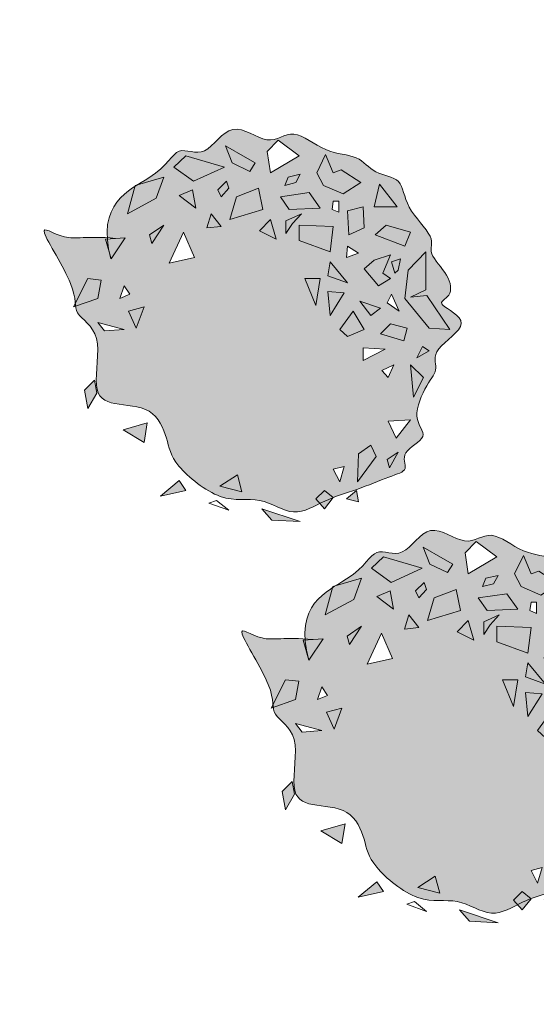
# Model space of a CAD drawing. Units: metres. Extents: x 4298.5 to 4325.2, y 2075 to 2095.8.
# Tile 23 of 35: x 4318.327 to 4319.132, y 2078.198 to 2079.73. Entities that reach past the tile are written whole.
import ezdxf

# ---------------------------------------------------------------- set-up
doc = ezdxf.new("R2010")
doc.units = ezdxf.units.M
doc.layers.add('A-ANNO-DIMS', color=2, linetype='Continuous', lineweight=18)
doc.layers.add('L-PLNT', color=94, linetype='Continuous', lineweight=13)
doc.layers.add('L-PLNT-PATT', color=116, linetype='Continuous', lineweight=13, true_color=0x13823e)
doc.styles.get("Standard").update_dxf_attribs({"font": 'arial.ttf'})
doc.dimstyles.get("Standard").update_dxf_attribs({"dimtxt": 0.18, "dimasz": 0.18, "dimexe": 0.18, "dimexo": 0.0625, "dimgap": 0.09, "dimtad": 0, "dimtih": 1, "dimtoh": 1, "dimdec": 4, "dimzin": 0, "dimdsep": 46, "dimtxsty": 'Standard', "dimcen": 0.09, "dimadec": 0, "dimazin": 0, "dimtfac": 1, "dimtdec": 4, "dimtofl": 0, "dimtmove": 0, "dimatfit": 3, "dimfxl": 1, "dimtolj": 1, "dimtzin": 0, "dimarcsym": 0})

# ---------------------------------------------------------------- blocks, each defined once
blk = doc.blocks.new('*U9')
for points in [[(-2.003, 11.656), (-1.598, 10.618), (-0.518, 10.099), (-0.181, 10.618), (-0.788, 10.964)], [(1.237, 12.003), (0.562, 11.31), (0.764, 10.013), (2.519, 11.051)], [(-4.432, 11.051), (-5.175, 10.359), (-3.96, 9.493), (-2.07, 10.359)], [(4.139, 11.137), (3.599, 10.013), (4.004, 9.234), (5.218, 8.715), (6.298, 9.407), (5.083, 10.186), (4.611, 10.013)], [(-5.782, 9.753), (-7.537, 9.234), (-8.009, 7.504), (-6.255, 8.455)], [(2.586, 9.926), (1.844, 9.753), (1.642, 9.234), (2.316, 9.407)], [(-1.935, 9.493), (-2.475, 8.974), (-2.273, 8.542), (-1.8, 9.061)], [(0.022, 9.061), (-1.328, 8.542), (-1.733, 7.157), (0.292, 7.763)], [(7.446, 9.32), (7.108, 7.936), (8.525, 7.936)], [(-4.837, 8.628), (-3.825, 7.85), (-4.027, 8.974)], [(1.372, 8.542), (3.126, 8.801), (3.801, 7.85), (1.912, 7.763)], [(4.611, 8.282), (4.544, 7.763), (4.949, 7.59), (4.949, 8.282)], [(6.433, 7.936), (5.488, 7.676), (5.556, 6.206), (6.501, 6.638)], [(-2.88, 7.504), (-3.15, 6.638), (-2.273, 6.725)], [(1.709, 6.292), (1.709, 7.071), (2.654, 7.504), (2.114, 6.898)], [(-5.782, 6.811), (-6.659, 6.206), (-6.524, 5.687)], [(0.764, 7.157), (0.089, 6.465), (1.102, 5.946)], [(2.519, 6.811), (2.519, 5.86), (4.409, 5.167), (4.611, 6.725)], [(7.851, 6.811), (7.176, 6.206), (8.998, 5.514), (9.335, 6.379)], [(-4.567, 6.379), (-5.445, 4.475), (-3.892, 4.821)], [(-8.144, 6.033), (-9.359, 5.946), (-9.022, 4.735)], [(5.488, 5.514), (5.421, 4.821), (6.163, 5.081)], [(8.12, 4.994), (7.108, 4.648), (6.501, 4.129), (7.378, 3.091), (8.12, 3.524), (7.648, 3.87)], [(10.28, 5.167), (9.2, 4.043), (8.998, 2.312), (10.482, 0.495), (11.765, 0.409), (10.348, 2.485), (9.335, 2.399), (10.28, 2.831)], [(4.409, 4.562), (4.274, 3.697), (5.488, 3.264)], [(8.728, 4.735), (8.188, 4.562), (8.39, 3.87), (8.593, 4.043)], [(-11.316, 1.793), (-9.831, 2.312), (-9.629, 3.437), (-10.439, 3.524)], [(-8.212, 3.091), (-8.482, 2.312), (-7.874, 2.572)], [(3.531, 1.88), (2.856, 3.524), (3.801, 3.524)], [(4.274, 2.745), (5.286, 2.658), (4.409, 1.274)], [(8.188, 2.572), (7.918, 2.053), (8.66, 1.534)], [(7.513, 1.707), (6.906, 1.274), (6.231, 2.139)], [(-6.997, 1.793), (-7.942, 1.534), (-7.469, 0.495)], [(5.826, 1.534), (5.016, 0.409), (5.488, -0.024), (6.501, 0.409)], [(-8.212, 0.409), (-9.426, 0.322), (-9.831, 0.841)], [(8.12, 0.755), (7.513, 0.149), (8.93, -0.283), (9.133, 0.495)], [(7.783, -0.803), (6.433, -1.495), (6.433, -0.716)], [(10.078, -0.629), (9.74, -1.322), (10.482, -0.889)], [(8.323, -1.754), (7.985, -2.533), (7.581, -2.1)], [(9.335, -1.754), (9.538, -3.744), (10.145, -2.533)], [(-10.034, -2.706), (-10.641, -3.312), (-10.439, -4.436), (-9.899, -3.485)], [(-8.279, -5.734), (-6.794, -5.302), (-6.997, -6.513)], [(9.335, -5.129), (8.458, -6.253), (7.985, -5.215)], [(6.096, -8.935), (6.163, -7.205), (6.906, -6.686), (7.243, -7.378)], [(8.053, -8.07), (8.593, -7.118), (7.918, -7.551)], [(5.286, -7.984), (4.611, -8.157), (5.016, -8.935)], [(-4.837, -8.849), (-4.432, -9.454), (-5.985, -9.801)], [(-2.34, -9.195), (-1.26, -8.503), (-0.99, -9.541)], [(4.071, -9.454), (3.531, -9.974), (4.071, -10.579), (4.611, -9.887)], [(6.028, -9.454), (5.421, -9.974), (6.163, -10.147)], [(-2.543, -10.06), (-3.015, -10.233), (-1.8, -10.666)], [(0.224, -10.579), (0.832, -11.272), (2.586, -11.358)]]:
    blk.add_lwpolyline(points, close=True)
blk = doc.blocks.new('*D47')
at = {"layer": 'A-ANNO-DIMS', "color": 0, "lineweight": -2, "transparency": 16777216}
for p, q in [((4300.4306, 2084.4956), (4300.4306, 2074.9896)), ((4322.8106, 2084.4956), (4322.8106, 2074.9896)), ((4300.6106, 2075.1696), (4311.2252, 2075.1696)), ((4322.6306, 2075.1696), (4312.016, 2075.1696))]:
    blk.add_line(p, q, dxfattribs=at)
at = {"layer": 'A-ANNO-DIMS', "color": 0, "transparency": 16777216}
for points in [[(4300.6106, 2075.1996), (4300.6106, 2075.1396), (4300.4306, 2075.1696)], [(4322.6306, 2075.1996), (4322.6306, 2075.1396), (4322.8106, 2075.1696)]]:
    blk.add_solid(points, dxfattribs=at)
at = {"layer": 'Defpoints', "color": 0, "transparency": 16777216}
for p in [(4300.4306, 2084.5581), (4322.8106, 2084.5581), (4322.8106, 2075.1696)]:
    blk.add_point(p, dxfattribs=at)
at = {"layer": 'A-ANNO-DIMS', "color": 0, "transparency": 16777216, "insert": (4311.6206, 2075.1696), "char_height": 0.18, "attachment_point": 5}
blk.add_mtext('\\A1;22.38', dxfattribs=at)
blk = doc.blocks.new('*D48')
at = {"layer": 'A-ANNO-DIMS', "color": 0, "lineweight": -2, "transparency": 16777216}
for p, q in [((4310.1831, 2094.4781), (4324.7671, 2094.4781)), ((4324.5871, 2094.2981), (4324.5871, 2085.585)), ((4324.5871, 2076.5081), (4324.5871, 2085.2212)), ((4316.8731, 2076.3281), (4324.7671, 2076.3281))]:
    blk.add_line(p, q, dxfattribs=at)
at = {"layer": 'A-ANNO-DIMS', "color": 0, "transparency": 16777216}
for points in [[(4324.5571, 2094.2981), (4324.6171, 2094.2981), (4324.5871, 2094.4781)], [(4324.5571, 2076.5081), (4324.6171, 2076.5081), (4324.5871, 2076.3281)]]:
    blk.add_solid(points, dxfattribs=at)
at = {"layer": 'Defpoints', "color": 0, "transparency": 16777216}
for p in [(4310.1206, 2094.4781), (4316.8106, 2076.3281), (4324.5871, 2076.3281)]:
    blk.add_point(p, dxfattribs=at)
at = {"layer": 'A-ANNO-DIMS', "color": 0, "transparency": 16777216, "insert": (4324.5871, 2085.4031), "char_height": 0.18, "attachment_point": 5}
blk.add_mtext('\\A1;18.15', dxfattribs=at)
blk = doc.blocks.new('*D79')
at = {"layer": 'A-ANNO-DIMS', "color": 0, "lineweight": -2, "transparency": 16777216}
for p, q in [((4313.4743, 2079.7393), (4313.4743, 2079.9193)), ((4313.3843, 2079.8293), (4313.5643, 2079.8293)), ((4320.4622, 2076.981), (4318.0084, 2077.9812)), ((4320.6422, 2076.981), (4320.4622, 2076.981))]:
    blk.add_line(p, q, dxfattribs=at)
at = {"layer": 'A-ANNO-DIMS', "color": 0, "transparency": 16777216}
blk.add_solid([(4318.0197, 2078.009), (4317.9971, 2077.9534), (4317.8417, 2078.0491)], dxfattribs=at)
at = {"layer": 'Defpoints', "color": 0, "transparency": 16777216}
for p in [(4313.4743, 2079.8293), (4317.8417, 2078.0491)]:
    blk.add_point(p, dxfattribs=at)
at = {"layer": 'A-ANNO-DIMS', "color": 0, "transparency": 16777216, "insert": (4321.3169, 2076.981), "char_height": 0.18, "attachment_point": 5}
blk.add_mtext('\\A1;2X R4.716', dxfattribs=at)

msp = doc.modelspace()

# ---------------------------------------------------------------- hatches: boundary and pattern name
at = {"layer": 'L-PLNT-PATT'}
h = msp.add_hatch(color=256, dxfattribs=at)
h.dxf.hatch_style = 1
edge = h.paths.add_edge_path()
edge.add_spline(control_points=[(4318.7946, 2078.9772), (4318.7972, 2078.9785), (4318.8158, 2078.9878), (4318.8516, 2078.9976), (4318.9061, 2079.0208), (4318.9355, 2079.0284), (4318.9167, 2079.0569), (4318.9693, 2079.0811), (4318.9356, 2079.1074), (4318.9626, 2079.1671), (4318.9813, 2079.1866), (4318.9647, 2079.2151), (4319.0389, 2079.26), (4318.969, 2079.2895), (4319.0017, 2079.2972), (4318.9977, 2079.3323), (4318.9596, 2079.3689), (4318.9782, 2079.3883), (4318.9251, 2079.4393), (4318.9251, 2079.4853), (4318.8773, 2079.4887), (4318.8568, 2079.5206), (4318.8036, 2079.5206), (4318.7513, 2079.5659), (4318.7165, 2079.5288), (4318.6558, 2079.5797), (4318.6159, 2079.5096), (4318.5713, 2079.5396), (4318.557, 2079.5002), (4318.5167, 2079.4772), (4318.5103, 2079.4732)], knot_values=[0.818571, 0.818571, 0.818571, 0.818571, 0.97924, 1.97924, 2.97924, 3.97924, 4.97924, 5.97924, 6.97924, 7.97924, 8.97924, 9.97924, 10.97924, 11.97924, 12.97924, 13.97924, 14.97924, 15.97924, 16.97924, 17.97924, 18.97924, 19.97924, 20.97924, 21.97924, 22.97924, 23.97924, 24.97924, 25.97924, 26.97924, 27.16067, 27.16067, 27.16067, 27.16067], degree=3, periodic=0)
edge.add_line((4318.5103, 2079.4732), (4318.5516, 2079.4854))
edge.add_line((4318.5516, 2079.4854), (4318.5396, 2079.4524))
edge.add_line((4318.5396, 2079.4524), (4318.495, 2079.4283))
edge.add_line((4318.495, 2079.4283), (4318.5067, 2079.4709))
edge.add_spline(control_points=[(4318.5067, 2079.4709), (4318.484, 2079.4562), (4318.4607, 2079.4353), (4318.4635, 2079.3909)], knot_values=[0.141368, 0.141368, 0.141368, 0.141368, 0.783694, 0.783694, 0.783694, 0.783694], degree=3, periodic=0)
edge.add_spline(control_points=[(4318.4635, 2079.3909), (4318.4674, 2079.3906), (4318.4717, 2079.3903), (4318.4762, 2079.3898)], knot_values=[40.901028, 40.901028, 40.901028, 40.901028, 41, 41, 41, 41], degree=3, periodic=0)
edge.add_line((4318.4762, 2079.3898), (4318.4916, 2079.3909))
edge.add_line((4318.4916, 2079.3909), (4318.4693, 2079.358))
edge.add_line((4318.4693, 2079.358), (4318.4608, 2079.3887))
edge.add_line((4318.4608, 2079.3887), (4318.4636, 2079.3889))
edge.add_spline(control_points=[(4318.4636, 2079.3889), (4318.4635, 2079.3896), (4318.4635, 2079.3902), (4318.4635, 2079.3909)], knot_values=[0.13204, 0.13204, 0.13204, 0.13204, 0.141368, 0.141368, 0.141368, 0.141368], degree=3, periodic=0)
edge.add_spline(control_points=[(4318.4635, 2079.3909), (4318.4272, 2079.3932), (4318.3956, 2079.3834), (4318.3436, 2079.4253), (4318.4107, 2079.3228), (4318.413, 2079.2959), (4318.4137, 2079.2885)], knot_values=[37.439141, 37.439141, 37.439141, 37.439141, 38.340169, 39.340169, 40.340169, 40.901028, 40.901028, 40.901028, 40.901028], degree=3, periodic=0)
edge.add_line((4318.4137, 2079.2885), (4318.4333, 2079.3272))
edge.add_line((4318.4333, 2079.3272), (4318.4539, 2079.325))
edge.add_line((4318.4539, 2079.325), (4318.4488, 2079.2964))
edge.add_line((4318.4488, 2079.2964), (4318.4141, 2079.2843))
edge.add_spline(control_points=[(4318.4141, 2079.2843), (4318.4146, 2079.2804), (4318.4177, 2079.2668), (4318.4591, 2079.2459), (4318.4376, 2079.1486), (4318.4698, 2079.1297), (4318.5361, 2079.1297), (4318.5588, 2079.076), (4318.5623, 2079.0405), (4318.6433, 2078.9745), (4318.7016, 2078.9912), (4318.752, 2078.9544), (4318.7811, 2078.9703), (4318.7946, 2078.9772)], knot_values=[27.16067, 27.16067, 27.16067, 27.16067, 27.490087, 28.490087, 29.490087, 30.490087, 31.490087, 32.490087, 33.490087, 34.490087, 35.490087, 36.490087, 37.329418, 37.329418, 37.329418, 37.329418], degree=3, periodic=0)
edge.add_line((4318.7946, 2078.9772), (4318.7882, 2078.9843))
edge.add_line((4318.7882, 2078.9843), (4318.8019, 2078.9976))
edge.add_line((4318.8019, 2078.9976), (4318.8156, 2078.9865))
h.paths.add_polyline_path([(4318.771, 2079.3272), (4318.795, 2079.3272), (4318.7882, 2079.2854)], flags=16)
h.paths.add_polyline_path([(4318.807, 2079.3074), (4318.8327, 2079.3052), (4318.8105, 2079.27)], flags=16)
h.paths.add_polyline_path([(4318.5996, 2079.3601), (4318.5602, 2079.3514), (4318.5825, 2079.3997)], flags=16)
h.paths.add_polyline_path([(4318.7265, 2079.3887), (4318.7007, 2079.4019), (4318.7179, 2079.4195)], flags=16)
h.paths.add_polyline_path([(4318.807, 2079.3316), (4318.8105, 2079.3536), (4318.8379, 2079.3206)], flags=16)
h.paths.add_polyline_path([(4318.8259, 2079.2481), (4318.8465, 2079.2766), (4318.8636, 2079.2481), (4318.8379, 2079.2371)], flags=16)
h.paths.add_polyline_path([(4318.7625, 2079.3865), (4318.7625, 2079.4107), (4318.8156, 2079.4085), (4318.8105, 2079.3689)], flags=16)
h.paths.add_polyline_path([(4318.7419, 2079.3975), (4318.7419, 2079.4173), (4318.7659, 2079.4283), (4318.7522, 2079.4129)], flags=16)
h.paths.add_polyline_path([(4318.6407, 2079.4085), (4318.6185, 2079.4063), (4318.6253, 2079.4283)], flags=16)
h.paths.add_polyline_path([(4318.6545, 2079.4195), (4318.6647, 2079.4547), (4318.699, 2079.4678), (4318.7059, 2079.4349)], flags=16)
h.paths.add_polyline_path([(4318.5207, 2079.2832), (4318.5088, 2079.2503), (4318.4967, 2079.2766)], flags=16)
h.paths.add_polyline_path([(4318.8567, 2079.292), (4318.8893, 2079.281), (4318.8739, 2079.27)], flags=16)
h.paths.add_polyline_path([(4318.8362, 2079.3601), (4318.8379, 2079.3777), (4318.855, 2079.3667)], flags=16)
h.paths.add_polyline_path([(4318.747, 2079.4349), (4318.7333, 2079.4547), (4318.7779, 2079.4612), (4318.795, 2079.4371)], flags=16)
h.paths.add_polyline_path([(4318.8619, 2079.2195), (4318.8962, 2079.2173), (4318.8619, 2079.1997)], flags=16)
h.paths.add_polyline_path([(4318.4985, 2079.303), (4318.483, 2079.2964), (4318.4899, 2079.3162)], flags=16)
h.paths.add_polyline_path([(4318.6013, 2079.4371), (4318.5756, 2079.4568), (4318.5962, 2079.4656)], flags=16)
h.paths.add_polyline_path([(4318.5328, 2079.3821), (4318.5293, 2079.3953), (4318.5516, 2079.4107)], flags=16)
h.paths.add_polyline_path([(4318.6407, 2079.4547), (4318.6356, 2079.4656), (4318.6493, 2079.4788), (4318.6528, 2079.4678)], flags=16)
h.paths.add_polyline_path([(4318.8636, 2079.3426), (4318.879, 2079.3557), (4318.9047, 2079.3645), (4318.8927, 2079.336), (4318.9047, 2079.3272), (4318.8859, 2079.3162)], flags=16)
h.paths.add_polyline_path([(4318.4899, 2079.2481), (4318.4591, 2079.2459), (4318.4488, 2079.259)], flags=16)
h.paths.add_polyline_path([(4318.8396, 2079.3953), (4318.8379, 2079.4327), (4318.8619, 2079.4393), (4318.8636, 2079.4063)], flags=16)
h.paths.add_polyline_path([(4318.8893, 2079.2415), (4318.9047, 2079.2569), (4318.9305, 2079.2503), (4318.9253, 2079.2305)], flags=16)
h.paths.add_polyline_path([(4318.8139, 2079.4349), (4318.8156, 2079.448), (4318.8242, 2079.448), (4318.8242, 2079.4305)], flags=16)
h.paths.add_polyline_path([(4318.7402, 2079.4722), (4318.7453, 2079.4854), (4318.7642, 2079.4898), (4318.7573, 2079.4766)], flags=16)
h.paths.add_polyline_path([(4318.8996, 2079.2898), (4318.9064, 2079.303), (4318.9184, 2079.2766)], flags=16)
h.paths.add_polyline_path([(4318.891, 2079.1843), (4318.9099, 2079.1931), (4318.9013, 2079.1733)], flags=16)
h.paths.add_polyline_path([(4318.6853, 2079.4942), (4318.6579, 2079.5074), (4318.6476, 2079.5337), (4318.6785, 2079.5162), (4318.6939, 2079.5074)], flags=16)
h.paths.add_polyline_path([(4318.7179, 2079.492), (4318.7127, 2079.525), (4318.7299, 2079.5426), (4318.7625, 2079.5184)], flags=16)
h.paths.add_polyline_path([(4318.5979, 2079.4788), (4318.567, 2079.5008), (4318.5859, 2079.5184), (4318.6459, 2079.5008)], flags=16)
h.paths.add_polyline_path([(4318.8807, 2079.3953), (4318.8979, 2079.4107), (4318.9356, 2079.3997), (4318.927, 2079.3777)], flags=16)
h.paths.add_polyline_path([(4318.8002, 2079.4722), (4318.7899, 2079.492), (4318.8036, 2079.5206), (4318.8156, 2079.492), (4318.8276, 2079.4964), (4318.8584, 2079.4766), (4318.831, 2079.459)], flags=16)
h.paths.add_polyline_path([(4318.9116, 2079.336), (4318.9064, 2079.3536), (4318.9202, 2079.358), (4318.9167, 2079.3404)], flags=16)
h.paths.add_polyline_path([(4318.927, 2079.2964), (4318.9322, 2079.3404), (4318.9596, 2079.3689), (4318.9596, 2079.3096), (4318.9356, 2079.2986), (4318.9613, 2079.3008), (4318.9973, 2079.2481), (4318.9647, 2079.2503)], flags=16)
h.paths.add_polyline_path([(4318.6665, 2079.0217), (4318.6733, 2078.9953), (4318.639, 2079.0041)], flags=16)
h.paths.add_polyline_path([(4318.879, 2079.4393), (4318.8876, 2079.4744), (4318.915, 2079.4393)], flags=16)
h.paths.add_polyline_path([(4318.9356, 2079.1931), (4318.9562, 2079.1733), (4318.9407, 2079.1426)], flags=16)
h.paths.add_polyline_path([(4318.9459, 2079.2041), (4318.9545, 2079.2217), (4318.9647, 2079.2151)], flags=16)
h.paths.add_polyline_path([(4318.8156, 2079.0305), (4318.8327, 2079.0349), (4318.8259, 2079.0107)], flags=16)
h.paths.add_polyline_path([(4318.9013, 2079.1052), (4318.9356, 2079.1074), (4318.9133, 2079.0789)], flags=16)
h.paths.add_polyline_path([(4318.855, 2079.0547), (4318.8739, 2079.0679), (4318.8824, 2079.0503), (4318.8533, 2079.0107)], flags=16)
h.paths.add_polyline_path([(4318.8996, 2079.0459), (4318.9167, 2079.0569), (4318.903, 2079.0327)], flags=16)
h = msp.add_hatch(color=256, dxfattribs=at)
h.dxf.hatch_style = 1
h.paths.add_polyline_path([(4318.8105, 2079.3689), (4318.8156, 2079.4085), (4318.7625, 2079.4107), (4318.7625, 2079.3865)])
h.paths.add_polyline_path([(4318.8567, 2079.292), (4318.8739, 2079.27), (4318.8893, 2079.281)])
h.paths.add_polyline_path([(4318.8379, 2079.4327), (4318.8396, 2079.3953), (4318.8636, 2079.4063), (4318.8619, 2079.4393)])
h.paths.add_polyline_path([(4318.8584, 2079.4766), (4318.8276, 2079.4964), (4318.8156, 2079.492), (4318.8036, 2079.5206), (4318.7899, 2079.492), (4318.8002, 2079.4722), (4318.831, 2079.459)])
h.paths.add_polyline_path([(4318.7042, 2078.969), (4318.7196, 2078.9514), (4318.7642, 2078.9492)])
h.paths.add_polyline_path([(4318.6853, 2079.4942), (4318.6939, 2079.5074), (4318.6785, 2079.5162), (4318.6476, 2079.5337), (4318.6579, 2079.5074)])
h.paths.add_polyline_path([(4318.5859, 2079.5184), (4318.567, 2079.5008), (4318.5979, 2079.4788), (4318.6459, 2079.5008)])
h.paths.add_polyline_path([(4318.6647, 2079.4547), (4318.6545, 2079.4195), (4318.7059, 2079.4349), (4318.699, 2079.4678)])
h.paths.add_polyline_path([(4318.6528, 2079.4678), (4318.6493, 2079.4788), (4318.6356, 2079.4656), (4318.6407, 2079.4547)])
h.paths.add_polyline_path([(4318.6253, 2079.4283), (4318.6185, 2079.4063), (4318.6407, 2079.4085)])
h.paths.add_polyline_path([(4318.6013, 2079.4371), (4318.5962, 2079.4656), (4318.5756, 2079.4568)])
h.paths.add_polyline_path([(4318.507, 2079.4722), (4318.495, 2079.4283), (4318.5396, 2079.4524), (4318.5516, 2079.4854)])
h.paths.add_polyline_path([(4318.5516, 2079.4107), (4318.5293, 2079.3953), (4318.5328, 2079.3821)])
h.paths.add_polyline_path([(4318.4608, 2079.3887), (4318.4693, 2079.358), (4318.4916, 2079.3909)])
h.paths.add_polyline_path([(4318.411, 2079.2832), (4318.4488, 2079.2964), (4318.4539, 2079.325), (4318.4333, 2079.3272)])
h.paths.add_polyline_path([(4318.5207, 2079.2832), (4318.4967, 2079.2766), (4318.5088, 2079.2503)])
h.paths.add_polyline_path([(4318.447, 2079.1492), (4318.4436, 2079.169), (4318.4282, 2079.1536), (4318.4333, 2079.125)])
h.paths.add_polyline_path([(4318.5259, 2079.103), (4318.4882, 2079.092), (4318.5207, 2079.0723)])
h.paths.add_polyline_path([(4318.5465, 2078.9887), (4318.5859, 2078.9976), (4318.5756, 2079.0129)])
h.paths.add_polyline_path([(4318.6665, 2079.0217), (4318.639, 2079.0041), (4318.6733, 2078.9953)])
h.paths.add_polyline_path([(4318.8019, 2078.9976), (4318.7882, 2078.9843), (4318.8019, 2078.969), (4318.8156, 2078.9866)])
h.paths.add_polyline_path([(4318.8824, 2079.0503), (4318.8739, 2079.0679), (4318.855, 2079.0547), (4318.8533, 2079.0107)])
h.paths.add_polyline_path([(4318.8516, 2078.9976), (4318.8362, 2078.9843), (4318.855, 2078.98)])
h.paths.add_polyline_path([(4318.8996, 2079.0459), (4318.903, 2079.0327), (4318.9167, 2079.0569)])
h.paths.add_polyline_path([(4318.9407, 2079.1426), (4318.9562, 2079.1733), (4318.9356, 2079.1931)])
h.paths.add_polyline_path([(4318.8259, 2079.2481), (4318.8379, 2079.2371), (4318.8636, 2079.2481), (4318.8465, 2079.2766)])
h.paths.add_polyline_path([(4318.9647, 2079.2503), (4318.9973, 2079.2481), (4318.9613, 2079.3008), (4318.9356, 2079.2986), (4318.9596, 2079.3096), (4318.9596, 2079.3689), (4318.9322, 2079.3404), (4318.927, 2079.2964)])
h.paths.add_polyline_path([(4318.9047, 2079.2569), (4318.8893, 2079.2415), (4318.9253, 2079.2305), (4318.9305, 2079.2503)])
h.paths.add_polyline_path([(4318.9647, 2079.2151), (4318.9545, 2079.2217), (4318.9459, 2079.2041)])
h.paths.add_polyline_path([(4318.9047, 2079.3645), (4318.879, 2079.3557), (4318.8636, 2079.3426), (4318.8859, 2079.3162), (4318.9047, 2079.3272), (4318.8927, 2079.336)])
h.paths.add_polyline_path([(4318.9064, 2079.3536), (4318.9116, 2079.336), (4318.9167, 2079.3404), (4318.9202, 2079.358)])
h.paths.add_polyline_path([(4318.927, 2079.3777), (4318.9356, 2079.3997), (4318.8979, 2079.4107), (4318.8807, 2079.3953)])
h.paths.add_polyline_path([(4318.8379, 2079.3206), (4318.8105, 2079.3536), (4318.807, 2079.3316)])
h.paths.add_polyline_path([(4318.795, 2079.3272), (4318.771, 2079.3272), (4318.7882, 2079.2854)])
h.paths.add_polyline_path([(4318.8327, 2079.3052), (4318.807, 2079.3074), (4318.8105, 2079.27)])
h.paths.add_polyline_path([(4318.795, 2079.4371), (4318.7779, 2079.4612), (4318.7333, 2079.4547), (4318.747, 2079.4349)])
h.paths.add_polyline_path([(4318.7522, 2079.4129), (4318.7659, 2079.4283), (4318.7419, 2079.4173), (4318.7419, 2079.3975)])
h.paths.add_polyline_path([(4318.7179, 2079.4195), (4318.7007, 2079.4019), (4318.7265, 2079.3887)])
h.paths.add_polyline_path([(4318.7573, 2079.4766), (4318.7642, 2079.4898), (4318.7453, 2079.4854), (4318.7402, 2079.4722)])
h.paths.add_polyline_path([(4318.8876, 2079.4744), (4318.879, 2079.4393), (4318.915, 2079.4393)])
h = msp.add_hatch(color=256, dxfattribs=at)
h.dxf.hatch_style = 1
edge = h.paths.add_edge_path()
edge.add_spline(control_points=[(4319.1026, 2078.3528), (4319.1051, 2078.3541), (4319.1238, 2078.3634), (4319.1596, 2078.3732), (4319.2141, 2078.3964), (4319.2435, 2078.4041), (4319.2247, 2078.4325), (4319.2773, 2078.4567), (4319.2436, 2078.483), (4319.2706, 2078.5428), (4319.2893, 2078.5622), (4319.2727, 2078.5907), (4319.3469, 2078.6356), (4319.277, 2078.6652), (4319.3097, 2078.6728), (4319.3057, 2078.7079), (4319.2676, 2078.7446), (4319.2862, 2078.7639), (4319.2331, 2078.8149), (4319.2331, 2078.8609), (4319.1852, 2078.8643), (4319.1648, 2078.8962), (4319.1116, 2078.8962), (4319.0593, 2078.9415), (4319.0245, 2078.9044), (4318.9638, 2078.9553), (4318.9239, 2078.8852), (4318.8793, 2078.9152), (4318.865, 2078.8758), (4318.8247, 2078.8528), (4318.8183, 2078.8488)], knot_values=[0.818571, 0.818571, 0.818571, 0.818571, 0.97924, 1.97924, 2.97924, 3.97924, 4.97924, 5.97924, 6.97924, 7.97924, 8.97924, 9.97924, 10.97924, 11.97924, 12.97924, 13.97924, 14.97924, 15.97924, 16.97924, 17.97924, 18.97924, 19.97924, 20.97924, 21.97924, 22.97924, 23.97924, 24.97924, 25.97924, 26.97924, 27.16067, 27.16067, 27.16067, 27.16067], degree=3, periodic=0)
edge.add_line((4318.8183, 2078.8488), (4318.8596, 2078.861))
edge.add_line((4318.8596, 2078.861), (4318.8476, 2078.8281))
edge.add_line((4318.8476, 2078.8281), (4318.803, 2078.8039))
edge.add_line((4318.803, 2078.8039), (4318.8147, 2078.8465))
edge.add_spline(control_points=[(4318.8147, 2078.8465), (4318.792, 2078.8318), (4318.7687, 2078.8109), (4318.7714, 2078.7665)], knot_values=[0.141368, 0.141368, 0.141368, 0.141368, 0.783694, 0.783694, 0.783694, 0.783694], degree=3, periodic=0)
edge.add_spline(control_points=[(4318.7714, 2078.7665), (4318.7754, 2078.7662), (4318.7797, 2078.7659), (4318.7842, 2078.7654)], knot_values=[40.901028, 40.901028, 40.901028, 40.901028, 41, 41, 41, 41], degree=3, periodic=0)
edge.add_line((4318.7842, 2078.7654), (4318.7996, 2078.7665))
edge.add_line((4318.7996, 2078.7665), (4318.7773, 2078.7336))
edge.add_line((4318.7773, 2078.7336), (4318.7688, 2078.7643))
edge.add_line((4318.7688, 2078.7643), (4318.7716, 2078.7645))
edge.add_spline(control_points=[(4318.7716, 2078.7645), (4318.7715, 2078.7652), (4318.7715, 2078.7658), (4318.7714, 2078.7665)], knot_values=[0.13204, 0.13204, 0.13204, 0.13204, 0.141368, 0.141368, 0.141368, 0.141368], degree=3, periodic=0)
edge.add_spline(control_points=[(4318.7714, 2078.7665), (4318.7352, 2078.7688), (4318.7036, 2078.759), (4318.6516, 2078.801), (4318.7187, 2078.6984), (4318.721, 2078.6716), (4318.7217, 2078.6641)], knot_values=[37.439141, 37.439141, 37.439141, 37.439141, 38.340169, 39.340169, 40.340169, 40.901028, 40.901028, 40.901028, 40.901028], degree=3, periodic=0)
edge.add_line((4318.7217, 2078.6641), (4318.7413, 2078.7028))
edge.add_line((4318.7413, 2078.7028), (4318.7619, 2078.7006))
edge.add_line((4318.7619, 2078.7006), (4318.7568, 2078.672))
edge.add_line((4318.7568, 2078.672), (4318.7221, 2078.6599))
edge.add_spline(control_points=[(4318.7221, 2078.6599), (4318.7226, 2078.656), (4318.7257, 2078.6424), (4318.767, 2078.6215), (4318.7456, 2078.5242), (4318.7778, 2078.5054), (4318.8441, 2078.5054), (4318.8668, 2078.4516), (4318.8703, 2078.4162), (4318.9513, 2078.3501), (4319.0096, 2078.3669), (4319.06, 2078.33), (4319.0891, 2078.3459), (4319.1026, 2078.3528)], knot_values=[27.16067, 27.16067, 27.16067, 27.16067, 27.490087, 28.490087, 29.490087, 30.490087, 31.490087, 32.490087, 33.490087, 34.490087, 35.490087, 36.490087, 37.329418, 37.329418, 37.329418, 37.329418], degree=3, periodic=0)
edge.add_line((4319.1026, 2078.3528), (4319.0962, 2078.36))
edge.add_line((4319.0962, 2078.36), (4319.1099, 2078.3732))
edge.add_line((4319.1099, 2078.3732), (4319.1236, 2078.3622))
h.paths.add_polyline_path([(4319.079, 2078.7028), (4319.103, 2078.7028), (4319.0962, 2078.6611)], flags=16)
h.paths.add_polyline_path([(4319.115, 2078.683), (4319.1407, 2078.6808), (4319.1185, 2078.6457)], flags=16)
h.paths.add_polyline_path([(4318.9076, 2078.7358), (4318.8682, 2078.727), (4318.8905, 2078.7753)], flags=16)
h.paths.add_polyline_path([(4319.0345, 2078.7643), (4319.0087, 2078.7775), (4319.0259, 2078.7951)], flags=16)
h.paths.add_polyline_path([(4319.115, 2078.7072), (4319.1185, 2078.7292), (4319.1459, 2078.6962)], flags=16)
h.paths.add_polyline_path([(4319.1339, 2078.6237), (4319.1544, 2078.6523), (4319.1716, 2078.6237), (4319.1459, 2078.6127)], flags=16)
h.paths.add_polyline_path([(4319.0705, 2078.7622), (4319.0705, 2078.7863), (4319.1236, 2078.7841), (4319.1185, 2078.7446)], flags=16)
h.paths.add_polyline_path([(4319.0499, 2078.7731), (4319.0499, 2078.7929), (4319.0739, 2078.8039), (4319.0602, 2078.7885)], flags=16)
h.paths.add_polyline_path([(4318.9487, 2078.7841), (4318.9265, 2078.7819), (4318.9333, 2078.8039)], flags=16)
h.paths.add_polyline_path([(4318.9625, 2078.7951), (4318.9727, 2078.8303), (4319.007, 2078.8435), (4319.0139, 2078.8105)], flags=16)
h.paths.add_polyline_path([(4318.8287, 2078.6589), (4318.8168, 2078.6259), (4318.8047, 2078.6523)], flags=16)
h.paths.add_polyline_path([(4319.1647, 2078.6676), (4319.1973, 2078.6567), (4319.1819, 2078.6457)], flags=16)
h.paths.add_polyline_path([(4319.1442, 2078.7358), (4319.1459, 2078.7534), (4319.163, 2078.7424)], flags=16)
h.paths.add_polyline_path([(4319.055, 2078.8105), (4319.0413, 2078.8303), (4319.0859, 2078.8369), (4319.103, 2078.8127)], flags=16)
h.paths.add_polyline_path([(4319.1699, 2078.5951), (4319.2042, 2078.5929), (4319.1699, 2078.5753)], flags=16)
h.paths.add_polyline_path([(4318.8065, 2078.6786), (4318.791, 2078.672), (4318.7979, 2078.6918)], flags=16)
h.paths.add_polyline_path([(4318.9093, 2078.8127), (4318.8836, 2078.8325), (4318.9042, 2078.8412)], flags=16)
h.paths.add_polyline_path([(4318.8408, 2078.7578), (4318.8373, 2078.7709), (4318.8596, 2078.7863)], flags=16)
h.paths.add_polyline_path([(4318.9487, 2078.8303), (4318.9436, 2078.8412), (4318.9573, 2078.8544), (4318.9607, 2078.8435)], flags=16)
h.paths.add_polyline_path([(4319.1716, 2078.7182), (4319.187, 2078.7314), (4319.2127, 2078.7402), (4319.2007, 2078.7116), (4319.2127, 2078.7028), (4319.1939, 2078.6918)], flags=16)
h.paths.add_polyline_path([(4318.7979, 2078.6237), (4318.767, 2078.6215), (4318.7568, 2078.6347)], flags=16)
h.paths.add_polyline_path([(4319.1476, 2078.7709), (4319.1459, 2078.8083), (4319.1699, 2078.8149), (4319.1716, 2078.7819)], flags=16)
h.paths.add_polyline_path([(4319.1973, 2078.6171), (4319.2127, 2078.6325), (4319.2384, 2078.6259), (4319.2333, 2078.6061)], flags=16)
h.paths.add_polyline_path([(4319.1219, 2078.8105), (4319.1236, 2078.8237), (4319.1322, 2078.8237), (4319.1322, 2078.8061)], flags=16)
h.paths.add_polyline_path([(4319.0482, 2078.8479), (4319.0533, 2078.861), (4319.0722, 2078.8654), (4319.0653, 2078.8522)], flags=16)
h.paths.add_polyline_path([(4319.2076, 2078.6655), (4319.2144, 2078.6786), (4319.2264, 2078.6523)], flags=16)
h.paths.add_polyline_path([(4319.199, 2078.56), (4319.2179, 2078.5688), (4319.2093, 2078.549)], flags=16)
h.paths.add_polyline_path([(4318.9933, 2078.8698), (4318.9659, 2078.883), (4318.9556, 2078.9094), (4318.9865, 2078.8918), (4319.0019, 2078.883)], flags=16)
h.paths.add_polyline_path([(4319.0259, 2078.8676), (4319.0207, 2078.9006), (4319.0379, 2078.9182), (4319.0705, 2078.894)], flags=16)
h.paths.add_polyline_path([(4318.9059, 2078.8544), (4318.875, 2078.8764), (4318.8939, 2078.894), (4318.9539, 2078.8764)], flags=16)
h.paths.add_polyline_path([(4319.1887, 2078.7709), (4319.2059, 2078.7863), (4319.2436, 2078.7753), (4319.235, 2078.7534)], flags=16)
h.paths.add_polyline_path([(4319.1082, 2078.8479), (4319.0979, 2078.8676), (4319.1116, 2078.8962), (4319.1236, 2078.8676), (4319.1356, 2078.872), (4319.1664, 2078.8522), (4319.139, 2078.8347)], flags=16)
h.paths.add_polyline_path([(4319.2196, 2078.7116), (4319.2144, 2078.7292), (4319.2282, 2078.7336), (4319.2247, 2078.716)], flags=16)
h.paths.add_polyline_path([(4319.235, 2078.672), (4319.2401, 2078.716), (4319.2676, 2078.7446), (4319.2676, 2078.6852), (4319.2436, 2078.6742), (4319.2693, 2078.6764), (4319.3053, 2078.6237), (4319.2727, 2078.6259)], flags=16)
h.paths.add_polyline_path([(4318.9745, 2078.3973), (4318.9813, 2078.371), (4318.947, 2078.3798)], flags=16)
h.paths.add_polyline_path([(4319.187, 2078.8149), (4319.1956, 2078.85), (4319.223, 2078.8149)], flags=16)
h.paths.add_polyline_path([(4319.2436, 2078.5688), (4319.2642, 2078.549), (4319.2487, 2078.5182)], flags=16)
h.paths.add_polyline_path([(4319.2539, 2078.5797), (4319.2625, 2078.5973), (4319.2727, 2078.5907)], flags=16)
h.paths.add_polyline_path([(4319.1236, 2078.4061), (4319.1407, 2078.4105), (4319.1339, 2078.3864)], flags=16)
h.paths.add_polyline_path([(4319.2093, 2078.4808), (4319.2436, 2078.483), (4319.2213, 2078.4545)], flags=16)
h.paths.add_polyline_path([(4319.163, 2078.4303), (4319.1819, 2078.4435), (4319.1904, 2078.4259), (4319.1613, 2078.3864)], flags=16)
h.paths.add_polyline_path([(4319.2076, 2078.4215), (4319.2247, 2078.4325), (4319.211, 2078.4083)], flags=16)
h = msp.add_hatch(color=256, dxfattribs=at)
h.dxf.hatch_style = 1
h.paths.add_polyline_path([(4319.1185, 2078.7446), (4319.1236, 2078.7841), (4319.0705, 2078.7863), (4319.0705, 2078.7622)])
h.paths.add_polyline_path([(4319.1647, 2078.6676), (4319.1819, 2078.6457), (4319.1973, 2078.6567)])
h.paths.add_polyline_path([(4319.1459, 2078.8083), (4319.1476, 2078.7709), (4319.1716, 2078.7819), (4319.1699, 2078.8149)])
h.paths.add_polyline_path([(4319.1664, 2078.8522), (4319.1356, 2078.872), (4319.1236, 2078.8676), (4319.1116, 2078.8962), (4319.0979, 2078.8676), (4319.1082, 2078.8479), (4319.139, 2078.8347)])
h.paths.add_polyline_path([(4319.0122, 2078.3446), (4319.0276, 2078.327), (4319.0722, 2078.3248)])
h.paths.add_polyline_path([(4318.9933, 2078.8698), (4319.0019, 2078.883), (4318.9865, 2078.8918), (4318.9556, 2078.9094), (4318.9659, 2078.883)])
h.paths.add_polyline_path([(4318.8939, 2078.894), (4318.875, 2078.8764), (4318.9059, 2078.8544), (4318.9539, 2078.8764)])
h.paths.add_polyline_path([(4318.9727, 2078.8303), (4318.9625, 2078.7951), (4319.0139, 2078.8105), (4319.007, 2078.8435)])
h.paths.add_polyline_path([(4318.9607, 2078.8435), (4318.9573, 2078.8544), (4318.9436, 2078.8412), (4318.9487, 2078.8303)])
h.paths.add_polyline_path([(4318.9333, 2078.8039), (4318.9265, 2078.7819), (4318.9487, 2078.7841)])
h.paths.add_polyline_path([(4318.9093, 2078.8127), (4318.9042, 2078.8412), (4318.8836, 2078.8325)])
h.paths.add_polyline_path([(4318.815, 2078.8479), (4318.803, 2078.8039), (4318.8476, 2078.8281), (4318.8596, 2078.861)])
h.paths.add_polyline_path([(4318.8596, 2078.7863), (4318.8373, 2078.7709), (4318.8408, 2078.7578)])
h.paths.add_polyline_path([(4318.7688, 2078.7643), (4318.7773, 2078.7336), (4318.7996, 2078.7665)])
h.paths.add_polyline_path([(4318.719, 2078.6589), (4318.7568, 2078.672), (4318.7619, 2078.7006), (4318.7413, 2078.7028)])
h.paths.add_polyline_path([(4318.8287, 2078.6589), (4318.8047, 2078.6523), (4318.8168, 2078.6259)])
h.paths.add_polyline_path([(4318.755, 2078.5248), (4318.7516, 2078.5446), (4318.7362, 2078.5292), (4318.7413, 2078.5006)])
h.paths.add_polyline_path([(4318.8339, 2078.4786), (4318.7962, 2078.4677), (4318.8287, 2078.4479)])
h.paths.add_polyline_path([(4318.8545, 2078.3644), (4318.8939, 2078.3732), (4318.8836, 2078.3885)])
h.paths.add_polyline_path([(4318.9745, 2078.3973), (4318.947, 2078.3798), (4318.9813, 2078.371)])
h.paths.add_polyline_path([(4319.1099, 2078.3732), (4319.0962, 2078.36), (4319.1099, 2078.3446), (4319.1236, 2078.3622)])
h.paths.add_polyline_path([(4319.1904, 2078.4259), (4319.1819, 2078.4435), (4319.163, 2078.4303), (4319.1613, 2078.3864)])
h.paths.add_polyline_path([(4319.1596, 2078.3732), (4319.1442, 2078.36), (4319.163, 2078.3556)])
h.paths.add_polyline_path([(4319.2076, 2078.4215), (4319.211, 2078.4083), (4319.2247, 2078.4325)])
h.paths.add_polyline_path([(4319.2487, 2078.5182), (4319.2642, 2078.549), (4319.2436, 2078.5688)])
h.paths.add_polyline_path([(4319.1339, 2078.6237), (4319.1459, 2078.6127), (4319.1716, 2078.6237), (4319.1544, 2078.6523)])
h.paths.add_polyline_path([(4319.2727, 2078.6259), (4319.3053, 2078.6237), (4319.2693, 2078.6764), (4319.2436, 2078.6742), (4319.2676, 2078.6852), (4319.2676, 2078.7446), (4319.2401, 2078.716), (4319.235, 2078.672)])
h.paths.add_polyline_path([(4319.2127, 2078.6325), (4319.1973, 2078.6171), (4319.2333, 2078.6061), (4319.2384, 2078.6259)])
h.paths.add_polyline_path([(4319.2727, 2078.5907), (4319.2625, 2078.5973), (4319.2539, 2078.5797)])
h.paths.add_polyline_path([(4319.2127, 2078.7402), (4319.187, 2078.7314), (4319.1716, 2078.7182), (4319.1939, 2078.6918), (4319.2127, 2078.7028), (4319.2007, 2078.7116)])
h.paths.add_polyline_path([(4319.2144, 2078.7292), (4319.2196, 2078.7116), (4319.2247, 2078.716), (4319.2282, 2078.7336)])
h.paths.add_polyline_path([(4319.235, 2078.7534), (4319.2436, 2078.7753), (4319.2059, 2078.7863), (4319.1887, 2078.7709)])
h.paths.add_polyline_path([(4319.1459, 2078.6962), (4319.1185, 2078.7292), (4319.115, 2078.7072)])
h.paths.add_polyline_path([(4319.103, 2078.7028), (4319.079, 2078.7028), (4319.0962, 2078.6611)])
h.paths.add_polyline_path([(4319.1407, 2078.6808), (4319.115, 2078.683), (4319.1185, 2078.6457)])
h.paths.add_polyline_path([(4319.103, 2078.8127), (4319.0859, 2078.8369), (4319.0413, 2078.8303), (4319.055, 2078.8105)])
h.paths.add_polyline_path([(4319.0602, 2078.7885), (4319.0739, 2078.8039), (4319.0499, 2078.7929), (4319.0499, 2078.7731)])
h.paths.add_polyline_path([(4319.0259, 2078.7951), (4319.0087, 2078.7775), (4319.0345, 2078.7643)])
h.paths.add_polyline_path([(4319.0653, 2078.8522), (4319.0722, 2078.8654), (4319.0533, 2078.861), (4319.0482, 2078.8479)])
h.paths.add_polyline_path([(4319.1956, 2078.85), (4319.187, 2078.8149), (4319.223, 2078.8149)])

# ---------------------------------------------------------------- linework, layer by layer
at = {"layer": 'L-PLNT'}
for points in [[(4318.4693, 2079.358), (4318.4452, 2079.4445), (4318.5516, 2079.4854), (4318.5713, 2079.5396), (4318.6159, 2079.5096), (4318.6558, 2079.5797), (4318.7165, 2079.5288), (4318.7513, 2079.5659), (4318.8036, 2079.5206), (4318.8568, 2079.5206), (4318.8773, 2079.4887), (4318.9251, 2079.4853), (4318.9251, 2079.4393), (4318.9782, 2079.3883), (4318.9596, 2079.3689), (4318.9977, 2079.3323), (4319.0017, 2079.2972), (4318.969, 2079.2895), (4319.0389, 2079.26), (4318.9647, 2079.2151), (4318.9813, 2079.1866), (4318.9626, 2079.1671), (4318.9356, 2079.1074), (4318.9693, 2079.0811), (4318.9167, 2079.0569), (4318.9355, 2079.0284), (4318.9061, 2079.0208), (4318.8516, 2078.9976), (4318.8019, 2078.984), (4318.7548, 2078.9523), (4318.7016, 2078.9912), (4318.6433, 2078.9745), (4318.5623, 2079.0405), (4318.5588, 2079.076), (4318.5361, 2079.1297), (4318.4698, 2079.1297), (4318.4376, 2079.1486), (4318.4591, 2079.2459), (4318.4058, 2079.2729), (4318.4222, 2079.3052), (4318.3436, 2079.4253), (4318.3974, 2079.3819), (4318.4305, 2079.3943), (4318.4762, 2079.3898)], [(4318.7773, 2078.7336), (4318.7532, 2078.8201), (4318.8596, 2078.861), (4318.8793, 2078.9152), (4318.9239, 2078.8852), (4318.9638, 2078.9553), (4319.0245, 2078.9044), (4319.0593, 2078.9415), (4319.1116, 2078.8962), (4319.1648, 2078.8962), (4319.1852, 2078.8643), (4319.2331, 2078.8609), (4319.2331, 2078.8149), (4319.2862, 2078.7639), (4319.2676, 2078.7446), (4319.3057, 2078.7079), (4319.3097, 2078.6728), (4319.277, 2078.6652), (4319.3469, 2078.6356), (4319.2727, 2078.5907), (4319.2893, 2078.5622), (4319.2706, 2078.5428), (4319.2436, 2078.483), (4319.2773, 2078.4567), (4319.2247, 2078.4325), (4319.2435, 2078.4041), (4319.2141, 2078.3964), (4319.1596, 2078.3732), (4319.1099, 2078.3596), (4319.0628, 2078.3279), (4319.0096, 2078.3669), (4318.9513, 2078.3501), (4318.8703, 2078.4162), (4318.8668, 2078.4516), (4318.8441, 2078.5054), (4318.7778, 2078.5054), (4318.7456, 2078.5242), (4318.767, 2078.6215), (4318.7138, 2078.6485), (4318.7302, 2078.6808), (4318.6516, 2078.801), (4318.7054, 2078.7576), (4318.7385, 2078.77), (4318.7842, 2078.7654)]]:
    msp.add_open_spline(points, degree=3, dxfattribs=at)

# ---------------------------------------------------------------- block references
at = {"layer": 'L-PLNT', "xscale": 0.0254, "yscale": 0.0254, "zscale": 0.0254}
for p in [(4318.6985, 2079.2377), (4319.0065, 2078.6133)]:
    msp.add_blockref('*U9', p, dxfattribs=at)

# ---------------------------------------------------------------- dimensions: what is measured, and where the dimension line sits
at = {"layer": 'A-ANNO-DIMS'}
dim = msp.add_linear_dim(base=(4324.5871, 2076.3281), p1=(4310.1206, 2094.4781), p2=(4316.8106, 2076.3281), angle=90, dimstyle='Standard', override={"dimdec": 2, "dimlfac": 1, "dimrnd": 0, "dimzin": 0, "dimdsep": 46, "dimlunit": 2}, dxfattribs=at)
dim.commit()
dim.dimension.update_dxf_attribs({"geometry": '*D48', "text_midpoint": (4324.5871, 2085.4031)})
dim = msp.add_linear_dim(base=(4322.8106, 2075.1696), p1=(4300.4306, 2084.5581), p2=(4322.8106, 2084.5581), dimstyle='Standard', override={"dimdec": 2, "dimlfac": 1, "dimrnd": 0, "dimzin": 0, "dimdsep": 46, "dimlunit": 2}, dxfattribs=at)
dim.commit()
dim.dimension.update_dxf_attribs({"geometry": '*D47', "text_midpoint": (4311.6206, 2075.1696)})
dim = msp.add_radius_dim(center=(4313.4743, 2079.8293), mpoint=(4317.8417, 2078.0491), text='2X <>', dimstyle='Standard', override={"dimdec": 3, "dimlfac": 1, "dimrnd": 0, "dimzin": 0, "dimdsep": 46, "dimlunit": 2}, dxfattribs=at)
dim.commit()
dim.dimension.update_dxf_attribs({"geometry": '*D79', "text_midpoint": (4321.3169, 2076.981), "dimtype": 164})

doc.saveas('drawing.dxf')
